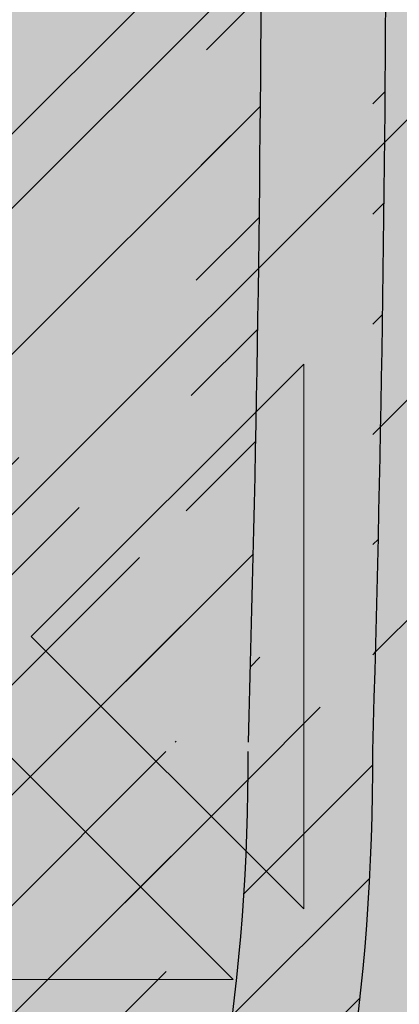
# Model space of a CAD drawing. Units: inches. Extents: x 844 to 2234, y 346 to 1084.
# Tile 11 of 93: x 1124.585 to 1125.555, y 691.183 to 693.702. Entities that reach past the tile are written whole.
import ezdxf

# ---------------------------------------------------------------- set-up
doc = ezdxf.new("R2010")
doc.units = ezdxf.units.IN
doc.header["$MEASUREMENT"] = 0
for name, color, linetype, lineweight in [('A-ANNO-DIMS', 2, 'Continuous', 18), ('furniture', 8, 'Continuous', 18), ('RA-AP-01$0$INT', 35, 'Continuous', 5)]:
    doc.layers.add(name, color=color, linetype=linetype, lineweight=lineweight)
doc.layers.add('RA-AP-01$0$FURN', color=3, linetype='Continuous')
doc.layers.add('RA-AP-01$0$WOOD', color=64, linetype='Continuous')
doc.styles.get("Standard").update_dxf_attribs({"font": 'arial.ttf'})
doc.dimstyles.get("Standard").update_dxf_attribs({"dimtxt": 6, "dimasz": 3, "dimexe": 0.18, "dimexo": 0.0625, "dimgap": 0.09, "dimtad": 0, "dimtih": 1, "dimtoh": 1, "dimdec": 1, "dimzin": 0, "dimdsep": 46, "dimlunit": 3, "dimtxsty": 'Standard', "dimblk": 'ARCHTICK', "dimcen": 0.09, "dimadec": 0, "dimazin": 0, "dimtfac": 1, "dimtdec": 1, "dimtofl": 0, "dimtmove": 0, "dimatfit": 3, "dimfxl": 1, "dimtolj": 1, "dimtzin": 0, "dimarcsym": 0})

# ---------------------------------------------------------------- blocks, each defined once
blk = doc.blocks.new('A$C18D01794')
at = {"layer": 'RA-AP-01$0$INT'}
h = blk.add_hatch(color=256, dxfattribs=at)
h.paths.add_polyline_path([(4.585917135068449, -6.356712009588271), (4.555206456959269, -6.35671200958746), (4.555206456959137, -6.387422687716308), (4.874495778835233, -6.706712009592356), (4.90520645695423, -6.676001331474049)])
h.paths.add_polyline_path([(5.255206456948813, -6.387422687716306), (5.255206456948682, -6.356712009605972), (5.224495778822613, -6.356712009605161), (4.905206456953498, -6.676001331474273), (4.935917135072151, -6.706712009592924)])
h.paths.add_polyline_path([(4.935917135072559, -6.706712009592068), (4.905206456953564, -6.737422687710376), (5.255206456951813, -7.087422687708613), (5.255206456951549, -7.026001331471008)])
h.paths.add_polyline_path([(4.555206456956399, -7.026001331471013), (4.555206456956134, -7.087422687708616), (4.905206456953821, -6.737422687710943), (4.874495778835166, -6.70671200959229)])
h = blk.add_hatch(color=256, dxfattribs=at)
h.paths.add_polyline_path([(4.585917135068448, -6.356712009588273), (4.614201406330596, -6.356712009589021), (4.668846067270487, -6.411356670531338), (4.723490728212344, -6.356712009591912), (4.771774999457151, -6.35671200959319), (4.826419660396886, -6.411356670535356), (4.862780050090322, -6.374996280843536), (4.844495778842715, -6.356712009595112), (4.862780050090411, -6.356712009595595), (4.905206456960182, -6.399138416468211), (4.947632863832445, -6.356712009597838), (4.965917135079675, -6.356712009598322), (4.947632863831759, -6.374996280845421), (4.983993253523576, -6.411356670538857), (5.038637914464627, -6.356712009600247), (5.08692218571208, -6.356712009601523), (5.141566846649976, -6.411356670541852), (5.196211507589851, -6.356712009604411), (5.224495778822615, -6.356712009605161), (4.905206456953975, -6.676001331473793)])
h.paths.add_polyline_path([(4.895206456956031, -6.637717060225675), (4.895206456958921, -6.528427738347902), (4.840561796018589, -6.583072399285802)], flags=16)
h.paths.add_polyline_path([(4.915206456955638, -6.637717060226121), (4.969851117895509, -6.583072399288678), (4.915206456957609, -6.528427738348344)], flags=16)
h.paths.add_polyline_path([(4.826419660395175, -6.568930263661755), (4.881064321335613, -6.514285602723745), (4.771774999456703, -6.514285602720857)], flags=16)
h.paths.add_polyline_path([(4.983993253519558, -6.568930263665262), (5.038637914460456, -6.514285602726792), (4.929348592581548, -6.514285602724816)], flags=16)
h.paths.add_polyline_path([(4.881064321336025, -6.494285602723742), (4.826419660397532, -6.439640941782821), (4.771774999457062, -6.494285602720859)], flags=16)
h.paths.add_polyline_path([(4.929348592582019, -6.494285602724817), (5.038637914460982, -6.494285602726792), (4.983993253522945, -6.439640941786327)], flags=16)
h.paths.add_polyline_path([(4.895206456960191, -6.480143467100443), (4.895206456962115, -6.407422687715913), (4.876922185715016, -6.389138416467584), (4.840561796021581, -6.425498806159401)], flags=16)
h.paths.add_polyline_path([(4.915206456958487, -6.480143467100889), (4.969851117899527, -6.425498806162279), (4.933490728206909, -6.389138416468043), (4.9152064569598, -6.40742268771434)], flags=16)
h.paths.add_polyline_path([(4.757632863832376, -6.480143467096812), (4.812277524772842, -6.425498806158772), (4.757632863834348, -6.370854145217844)], flags=16)
h.paths.add_polyline_path([(4.737632863832376, -6.480143467096286), (4.737632863834348, -6.370854145217375), (4.682988202893906, -6.425498806155385)], flags=16)
h.paths.add_polyline_path([(5.05278005008503, -6.480143467103376), (5.052780050087917, -6.370854145224413), (4.998135389146995, -6.425498806162908)], flags=16)
h.paths.add_polyline_path([(5.072780050085024, -6.480143467103744), (5.127424711025931, -6.42549880616527), (5.072780050087916, -6.370854145224832)], flags=16)
h.paths.add_polyline_path([(4.935917135072783, -6.706712009592292), (5.255206456948811, -6.387422687716309), (5.255206456948932, -6.415706958964177), (5.200561796010279, -6.470351619902839), (5.255206456949403, -6.524996280841948), (5.25520645694961, -6.5732805520894), (5.200561796009787, -6.627925213029239), (5.236922185702417, -6.664285602721864), (5.255206456949919, -6.646001331474357), (5.255206456949998, -6.664285602721898), (5.212780050078687, -6.706712009592262), (5.25520645695036, -6.749138416463932), (5.255206456950438, -6.767422687711313), (5.236922185702424, -6.749138416463297), (5.200561796009796, -6.785498806155928), (5.255206456950753, -6.840143467096874), (5.25520645695096, -6.888427738341682), (5.200561796010322, -6.943072399282328), (5.255206456951428, -6.997717060223427), (5.255206456951547, -7.026001331471006)])
h.paths.add_polyline_path([(5.042988202883395, -6.785498806155427), (5.097632863823085, -6.840143467095101), (5.097632863822622, -6.730854145216193)], flags=16)
h.paths.add_polyline_path([(5.028846067259663, -6.771356670531693), (5.083490728198774, -6.716712009592573), (4.974201406321001, -6.716712009593042)], flags=16)
h.paths.add_polyline_path([(5.117632863823087, -6.840143467095186), (5.172277524762331, -6.785498806155926), (5.11763286382262, -6.730854145216225)], flags=16)
h.paths.add_polyline_path([(5.08349072819877, -6.696712009593886), (5.028846067259652, -6.642067348654775), (4.974201406320998, -6.696712009593438)], flags=16)
h.paths.add_polyline_path([(5.131774999446817, -6.854285602718917), (5.186419660386065, -6.799640941779662), (5.241064321325782, -6.854285602719365)], flags=17)
h.paths.add_polyline_path([(5.131774999446228, -6.716712009592374), (5.186419660386065, -6.771356670532194), (5.222780050079488, -6.734996280838764), (5.204495778832781, -6.716712009592063)], flags=16)
h.paths.add_polyline_path([(5.097632863822613, -6.682569873970264), (5.097632863823061, -6.573280552091354), (5.042988202883383, -6.627925213031044)], flags=16)
h.paths.add_polyline_path([(5.131774999446899, -6.874285602718915), (5.241064321325809, -6.874285602719364), (5.186419660386591, -6.928930263658598)], flags=17)
h.paths.add_polyline_path([(5.131774999446226, -6.696712009594078), (5.204495778830767, -6.696712009594374), (5.22278005007868, -6.67842773834687), (5.186419660386049, -6.642067348654249)], flags=16)
h.paths.add_polyline_path([(5.11763286382262, -6.682569873970225), (5.17227752476232, -6.627925213030515), (5.117632863823064, -6.573280552091267)], flags=16)
h.paths.add_polyline_path([(5.186419660386069, -6.613783077405491), (5.241064321325754, -6.559138416465795), (5.131774999446791, -6.559138416466263)], flags=16)
h.paths.add_polyline_path([(5.131774999446872, -6.539138416466263), (5.24106432132578, -6.539138416465794), (5.186419660386554, -6.484493755526573)], flags=16)
h.paths.add_polyline_path([(5.255206456951811, -7.08742268770861), (5.255206456951895, -7.106712009588038), (4.555206456956052, -7.106712009588038), (4.555206456956136, -7.087422687708617), (4.905206456953973, -6.737422687710788)])
h.paths.add_polyline_path([(4.983993253513404, -6.8444937555241), (4.92934859257295, -6.899138416462108), (5.03863791445186, -6.899138416465014)], flags=16)
h.paths.add_polyline_path([(4.969851117889988, -6.83035161990006), (4.915206456952556, -6.775706958960171), (4.915206456949648, -6.884996280837944)], flags=16)
h.paths.add_polyline_path([(4.929348592572535, -6.919138416462105), (4.983993253511019, -6.973783077403037), (5.038637914451496, -6.919138416465012)], flags=16)
h.paths.add_polyline_path([(5.052780050074912, -6.93328055208906), (4.998135389134438, -6.987925213027088), (5.052780050072919, -7.042569873968025)], flags=16)
h.paths.add_polyline_path([(5.07278005007491, -6.933280552089588), (5.072780050072918, -7.042569873968497), (5.127424711013374, -6.987925213030498)], flags=16)
h.paths.add_polyline_path([(4.89520645695295, -6.775706958959721), (4.840561796013067, -6.830351619897157), (4.895206456950961, -6.884996280837494)], flags=16)
h.paths.add_polyline_path([(4.915206456948365, -6.933280552085403), (4.915206456946434, -7.006001331471951), (4.933490728192729, -7.024285602719066), (4.969851117886972, -6.987925213026453)], flags=16)
h.paths.add_polyline_path([(4.881064321327021, -6.899138416461022), (4.82641966038902, -6.84449375552057), (4.771774999448108, -6.899138416459029)], flags=16)
h.paths.add_polyline_path([(4.895206456950073, -6.933280552084951), (4.840561796009022, -6.987925213023558), (4.876922185700835, -7.024285602716997), (4.895206456948749, -7.006001331469487)], flags=16)
h.paths.add_polyline_path([(4.983993253510392, -7.0020673486505), (4.947632863816944, -7.038427738342319), (4.965917135064043, -7.05671200959023), (5.038637914448995, -7.056712009591555)], flags=16)
h.paths.add_polyline_path([(4.881064321326543, -6.91913841646102), (4.771774999447578, -6.919138416459031), (4.826419660385607, -6.973783077399508)], flags=16)
h.paths.add_polyline_path([(4.905206456946447, -7.014285602717636), (4.862780050074785, -7.056712009588352), (4.947632863816685, -7.056712009589775)], flags=16)
h.paths.add_polyline_path([(5.14156684663679, -7.002067348654549), (5.086922185696452, -7.056712009592438), (5.196211507574223, -7.056712009594425)], flags=16)
h.paths.add_polyline_path([(4.8264196603837, -7.002067348646972), (4.771774999442643, -7.056712009585575), (4.8444957788276, -7.056712009587508), (4.862780050075511, -7.038427738340416)], flags=16)
h.paths.add_polyline_path([(4.812277524760289, -6.98792521302292), (4.757632863822258, -6.933280552082447), (4.757632863819352, -7.042569873961408)], flags=16)
h.paths.add_polyline_path([(4.73763286382226, -6.933280552082079), (4.682988202881349, -6.987925213020536), (4.737632863819352, -7.04256987396099)], flags=16)
h.paths.add_polyline_path([(4.723490728195188, -7.056712009584289), (4.668846067257299, -7.002067348643949), (4.614201406317417, -7.056712009581383)], flags=16)
h.paths.add_polyline_path([(4.597632863829262, -6.706712009592262), (4.555206456957951, -6.664285602721896), (4.555206456958029, -6.646001331474357), (4.573490728205535, -6.664285602721864), (4.609851117898167, -6.627925213029238), (4.555206456958338, -6.573280552089402), (4.555206456958546, -6.524996280841952), (4.60985111789767, -6.470351619902839), (4.555206456959015, -6.415706958964177), (4.555206456959138, -6.387422687716309), (4.874495778835167, -6.70671200959229), (4.5552064569564, -7.026001331471015), (4.555206456956523, -6.997717060223433), (4.609851117897629, -6.94307239928233), (4.555206456956988, -6.888427738341681), (4.555206456957198, -6.840143467096881), (4.609851117898153, -6.78549880615593), (4.573490728205528, -6.749138416463297), (4.555206456957507, -6.76742268771132), (4.555206456957585, -6.749138416463933)])
h.paths.add_polyline_path([(4.712780050085332, -6.730854145216195), (4.712780050084863, -6.840143467095105), (4.767424711024555, -6.785498806155427)], flags=16)
h.paths.add_polyline_path([(4.726922185709173, -6.716712009592573), (4.781566846648288, -6.771356670531693), (4.836211507586949, -6.716712009593043)], flags=16)
h.paths.add_polyline_path([(4.692780050085327, -6.730854145216225), (4.638135389145619, -6.785498806155928), (4.692780050084865, -6.840143467095185)], flags=16)
h.paths.add_polyline_path([(4.726922185709182, -6.696712009593886), (4.836211507586949, -6.696712009593436), (4.7815668466483, -6.642067348654773)], flags=16)
h.paths.add_polyline_path([(4.678637914461726, -6.71671200959237), (4.605917135075169, -6.716712009592063), (4.587632863828464, -6.734996280838766), (4.623993253521887, -6.771356670532195)], flags=16)
h.paths.add_polyline_path([(4.712780050085336, -6.68256987397026), (4.767424711024568, -6.627925213031042), (4.71278005008489, -6.573280552091352)], flags=16)
h.paths.add_polyline_path([(4.678637914461726, -6.696712009594076), (4.623993253521899, -6.642067348654247), (4.587632863829271, -6.67842773834687), (4.605917135077185, -6.696712009594376)], flags=16)
h.paths.add_polyline_path([(4.692780050085336, -6.682569873970228), (4.692780050084889, -6.573280552091267), (4.638135389145632, -6.627925213030515)], flags=16)
h.paths.add_polyline_path([(4.623993253521885, -6.799640941779662), (4.678637914461131, -6.854285602718915), (4.56934859258217, -6.854285602719365)], flags=17)
h.paths.add_polyline_path([(4.623993253521901, -6.613783077405509), (4.678637914461158, -6.559138416466263), (4.569348592582195, -6.559138416465795)], flags=16)
h.paths.add_polyline_path([(4.678637914461051, -6.874285602718915), (4.623993253521361, -6.928930263658598), (4.569348592582143, -6.874285602719364)], flags=17)
h.paths.add_polyline_path([(4.678637914461076, -6.539138416466263), (4.623993253521399, -6.484493755526573), (4.569348592582167, -6.539138416465796)], flags=16)
h = blk.add_hatch(color=256, dxfattribs=at)
h.paths.add_polyline_path([(5.028846067259997, -6.642067348655121), (4.974201406321342, -6.696712009593783), (5.083490728199115, -6.69671200959423)])
h.paths.add_polyline_path([(4.974201406321344, -6.716712009593388), (5.028846067260004, -6.771356670532039), (5.083490728199117, -6.716712009592919)])
h.paths.add_polyline_path([(5.042988202883738, -6.785498806155768), (5.097632863823428, -6.840143467095449), (5.097632863822963, -6.73085414521654)])
h.paths.add_polyline_path([(5.117632863822961, -6.730854145216568), (5.117632863823428, -6.840143467095531), (5.172277524762674, -6.785498806156272)])
h.paths.add_polyline_path([(5.131774999446572, -6.716712009592718), (5.186419660386406, -6.77135667053254), (5.222780050079831, -6.734996280839116), (5.204495778833122, -6.716712009592409)])
h.paths.add_polyline_path([(5.236922185702764, -6.749138416463644), (5.200561796010139, -6.785498806156274), (5.255206456949971, -6.840143467096101), (5.255206456950271, -6.76742268771115)])
h.paths.add_polyline_path([(5.186419660386412, -6.799640941780006), (5.131774999447164, -6.854285602719262), (5.241064321326123, -6.854285602719711)])
h.paths.add_polyline_path([(5.131774999447238, -6.874285602719261), (5.186419660386934, -6.928930263658944), (5.241064321326153, -6.874285602719709)])
h.paths.add_polyline_path([(5.200561796010663, -6.943072399282675), (5.255206456949324, -6.997717060221329), (5.255206456949777, -6.888427738343558)])
h.paths.add_polyline_path([(5.21278005007903, -6.706712009592607), (5.255206456950223, -6.749138416463798), (5.255206456950696, -6.664285602721891)])
h.paths.add_polyline_path([(5.13177499944657, -6.696712009594424), (5.204495778831106, -6.696712009594723), (5.222780050079024, -6.678427738347219), (5.186419660386397, -6.642067348654592)])
h.paths.add_polyline_path([(5.117632863823405, -6.573280552091611), (5.117632863822955, -6.682569873970578), (5.172277524762665, -6.627925213030859)])
h.paths.add_polyline_path([(5.042988202883727, -6.627925213031387), (5.097632863822957, -6.682569873970603), (5.097632863823407, -6.573280552091697)])
h.paths.add_polyline_path([(5.131774999447135, -6.559138416466609), (5.186419660386394, -6.613783077405857), (5.241064321326097, -6.559138416466144)])
h.paths.add_polyline_path([(5.200561796010128, -6.627925213029584), (5.236922185702758, -6.664285602722211), (5.255206456950264, -6.646001331474705), (5.255206456949948, -6.573280552089752)])
h.paths.add_polyline_path([(5.186419660386895, -6.484493755526919), (5.131774999447213, -6.539138416466609), (5.241064321326127, -6.539138416466142)])
h.paths.add_polyline_path([(5.200561796010624, -6.470351619903183), (5.255206456949745, -6.524996280842298), (5.255206456949276, -6.415706958964523)])
for p, q in [((4.935917135072783, -6.706712009592292), (5.255206456951548, -7.026001331471007)), ((5.083490728198772, -6.716712009592574), (4.974201406321001, -6.716712009593042)), ((5.08349072819877, -6.716712009592578), (5.028846067259663, -6.771356670531693)), ((5.09763286382262, -6.730854145216195), (5.042988202883395, -6.785498806155425)), ((5.097632863823085, -6.840143467095105), (5.09763286382262, -6.730854145216195)), ((4.905206456953975, -6.737422687710788), (5.255206456951811, -7.087422687708611)), ((5.042988202883397, -6.785498806155427), (5.097632863823085, -6.840143467095105))]:
    blk.add_line(p, q, dxfattribs=at)
blk = doc.blocks.new('A$C32926AE1')
at = {"layer": 'RA-AP-01$0$FURN'}
h = blk.add_hatch(dxfattribs=at)
h.set_pattern_fill('ANSI31', color=256, scale=0.1, style=0)
h.set_pattern_definition([(45, (0, 0), (-0.0088388347648318, 0.0088388347648318), [])])
edge = h.paths.add_edge_path(flags=16)
edge.add_arc((4.904771284329206, 4.246793130718756), 0.2603971832811541, 75.22398030683196, 104.7760196931204)
edge.add_arc((4.904771284329206, 4.246793130718756), 0.2603971832811541, 75.223980306832, 104.77601969312039, ccw=False)
edge = h.paths.add_edge_path(flags=16)
edge.add_arc((4.904771284329206, 4.067062675376612), 0.2603971832811541, 255.2239803068796, 284.776019693168)
edge.add_arc((4.904771284329206, 4.067062675376612), 0.2603971832811541, 255.22398030687958, 284.77601969316805, ccw=False)
edge = h.paths.add_edge_path(flags=0)
edge.add_arc((4.904771284329206, 4.067062675376612), 0.2603971832811541, 255.2239803068796, 284.776019693168)
edge.add_arc((4.904771284329206, 4.067062675376612), 0.2603971832811541, 255.22398030687958, 284.77601969316805, ccw=False)
edge = h.paths.add_edge_path(flags=0)
edge.add_arc((4.904771284329206, 4.067062675376612), 0.2603971832811541, 255.2239803068796, 284.776019693168)
edge.add_arc((4.904771284329206, 4.067062675376612), 0.2603971832811541, 255.22398030687958, 284.77601969316805, ccw=False)
edge = h.paths.add_edge_path()
edge.add_arc((4.604388392048174, 4.588829985554312), 0.1599999999999918, 342.3781640246255, 354.4317409793762)
edge.add_arc((5.090145208887507, 4.43216705527679), 0.3503971832811637, 162.0091218307731, 180.3186872093483)
edge.add_arc((5.205154176610243, 4.588829985554953), 0.1599999999999917, 185.5682590208461, 197.6218359767349)
edge.add_arc((4.904771284329229, 4.246793130718735), 0.3503971832811761, 72.00912183053516, 107.9908781690354)
edge.add_arc((9.535952835716557, 4.28682295566602), 4.798342501046485, 178.2875002453811, 181.5576802719453)
edge.add_arc((4.719397359771122, 4.43216705527679), 0.3503971832811637, 359.6813127906516, 377.9908781692269)
edge.add_arc((9.535967292294904, 4.286822350292874), 4.778371420254705, 178.2965938931842, 181.5667745797229)
edge.add_arc((4.719397359771122, 4.43216705527679), 0.3303971832811637, 359.6813127906516, 377.9908781692269)
edge.add_arc((0.2735752763637294, 4.286822350292874), 4.7783714202547, 358.4332254202771, 361.7034061068158)
edge.add_arc((5.061434214606998, 4.732549947558029), 0.1600000000000254, 252.3781640250584, 264.4317409792362)
edge.add_arc((4.748108354051257, 4.732549947558012), 0.1600000000000541, 275.5682590208426, 287.6218359759532)
edge.add_arc((4.604388392048115, 4.588829985554317), 0.1800000000000505, 342.3567572500182, 349.3735009646207)
edge.add_arc((5.205154176610254, 4.588829985554976), 0.1800000000000069, 190.6264990356027, 197.6432427513933)
edge.add_arc((5.061434214607106, 4.732549947558013), 0.1800000000000424, 252.3567572496606, 259.3735009644582)
edge.add_arc((4.904771284329208, 4.246793130718737), 0.3303971832811676, 71.99844483668534, 108.0015551637021)
edge.add_arc((4.748108354051414, 4.732549947558045), 0.1800000000000547, 280.6264990355479, 287.6432427495938)
edge.add_arc((5.090145208887514, 4.432167055276789), 0.2803971832811691, 162.8706300666893, 180.816523289902)
edge.add_arc((4.719397359771136, 4.432167055276689), 0.2803971832811534, 359.183476710103, 377.1293699333214)
edge.add_arc((4.904771284329222, 4.246793130718737), 0.2803971832811769, 72.87063006672916, 107.1293699332334)
edge.add_arc((5.090145208887522, 4.432167055276788), 0.2603971832811776, 165.2239803068007, 180.9953123810312)
edge.add_arc((4.719397359771141, 4.432167055276699), 0.2603971832811458, 359.0046876189768, 374.7760196932087)
edge.add_arc((5.090145208887507, 4.43216705527679), 0.3303971832811637, 162.0091218307731, 180.3186872093483)
edge.add_arc((9.53595427642584, 4.285015535491528), 4.728345371032053, 178.265043920078, 181.5679956281801)
edge.add_arc((0.2735882922327999, 4.285015535491582), 4.728345371032045, 358.4320043718193, 361.7349560799204)
edge.add_arc((9.535953591267507, 4.284458026472751), 4.708343996644348, 178.2573054306777, 181.5704995759608)
edge.add_arc((0.273588977391114, 4.284458026472785), 4.708343996644358, 358.4295004240388, 361.7426945693213)
edge.add_arc((0.2735889773911131, 4.029397779622582), 4.708343996644359, 358.2573054306787, 361.5704995759613)
edge.add_arc((9.535953591267518, 4.029397779622618), 4.708343996644359, 178.4295004240391, 181.7426945693223)
edge.add_arc((0.2735882922327901, 4.028840270603786), 4.728345371032054, 358.2650439200796, 361.5679956281808)
edge.add_arc((9.53595427642584, 4.028840270603841), 4.728345371032054, 178.4320043718199, 181.7349560799219)
edge.add_arc((0.2735752763637302, 4.027033455802493), 4.778371420254699, 358.2965938931842, 361.5667745797229)
edge.add_arc((4.719397359771122, 3.881688750818578), 0.3303971832811637, 342.0091218307731, 360.3186872093484)
edge.add_arc((5.090145208887507, 3.881688750818578), 0.3303971832811637, 179.6813127906516, 197.9908781692269)
edge.add_arc((9.535967292294904, 4.027033455802493), 4.778371420254705, 178.433225420277, 181.7034061068158)
edge.add_arc((4.719397359771122, 3.881688750818578), 0.3503971832811637, 342.0091218307731, 360.3186872093484)
edge.add_arc((9.53595283571655, 4.027032850429349), 4.79834250104648, 178.4423197280546, 181.7124997546188)
edge.add_arc((4.719397359771141, 3.881688750818669), 0.2603971832811458, 345.2239803067913, 360.9953123810232)
edge.add_arc((5.090145208887522, 3.88168875081858), 0.2603971832811776, 179.0046876189687, 194.7760196931993)
edge.add_arc((4.904771284329222, 4.067062675376631), 0.2803971832811769, 252.8706300667665, 287.1293699332708)
edge.add_arc((4.719397359771136, 3.881688750818678), 0.2803971832811534, 342.8706300666787, 360.8165232898969)
edge.add_arc((5.090145208887514, 3.881688750818579), 0.2803971832811691, 179.183476710098, 197.1293699333106)
edge.add_arc((4.748108354051414, 3.581305858537323), 0.1800000000000547, 72.3567572504062, 79.37350096445199)
edge.add_arc((4.904771284329208, 4.067062675376631), 0.3303971832811676, 251.9984448362979, 288.0015551633146)
edge.add_arc((5.061434214607106, 3.581305858537355), 0.1800000000000424, 100.6264990355418, 107.6432427503394)
edge.add_arc((5.205154176610254, 3.725025820540392), 0.1800000000000069, 162.3567572486066, 169.3735009643972)
edge.add_arc((4.604388392048115, 3.725025820541051), 0.1800000000000505, 10.62649903537925, 17.64324274998182)
edge.add_arc((4.748108354051257, 3.581305858537356), 0.1600000000000541, 72.37816402404681, 84.43174097915735)
edge.add_arc((4.904771284329229, 4.067062675376632), 0.3503971832811761, 252.0091218309645, 287.9908781694648)
edge.add_arc((5.061434214606998, 3.581305858537339), 0.1600000000000254, 95.56825902076373, 107.6218359749416)
edge.add_arc((5.205154176610243, 3.725025820540414), 0.1599999999999917, 162.3781640232651, 174.4317409791539)
edge.add_arc((5.090145208887507, 3.881688750818578), 0.3503971832811637, 179.6813127906516, 197.9908781692269)
edge.add_arc((4.604388392048174, 3.725025820541056), 0.1599999999999918, 5.568259020623824, 17.62183597537444)
edge.add_arc((0.2735897329420762, 4.28682295566602), 4.798342501046482, 358.4423197280547, 361.7124997546188)
edge.add_arc((0.2735897329420691, 4.027032850429348), 4.798342501046489, 358.2875002453812, 361.5576802719453)
at = {"layer": 'RA-AP-01$0$WOOD'}
h = blk.add_hatch(color=256, dxfattribs=at)
h.dxf.hatch_style = 1
h.paths.add_polyline_path([(5.157430609644524, 4.573483066760929, -0.1009492694046607), (5.155401577623758, 4.593365984175333, -0.1842662638101597), (5.172249623284174, 4.638795604568598, 0.2056608120311276), (5.179560981299304, 4.661316324430096, 0.3614336704623542), (5.134352340494423, 4.706524965234944, 0.2056608120311297), (5.111831620632933, 4.699213607219793, -0.1842662638101113), (5.066402000239693, 4.682365561559342, -0.1055311479399994), (5.045656153913092, 4.68467289944697, 0.1567636581983829), (4.763886414745334, 4.684672899446966, -0.1055311479399895), (4.743140568418733, 4.68236556155934, -0.1842662638100833), (4.6977109480255, 4.69921360721979, 0.2056608120302612), (4.675190228164109, 4.706524965234949, 0.3614336704708441), (4.629981587358889, 4.66131632442871, 0.2056608120245944), (4.637292945374126, 4.638795604567974, -0.1842662638101024), (4.654140991034615, 4.59336598417475, -0.1009492694055169), (4.652111959013835, 4.573483066760181, 0.021410119221476), (4.629748025606143, 4.156712009541676, 0.0214101192214795), (4.652111959013809, 3.739940952323101, -0.1009492694059586), (4.654140991034615, 3.720058034908448, -0.1842662638100975), (4.637292945374126, 3.674628414515226, 0.2056608120245705), (4.629981587358889, 3.652107694654492, 0.3614336704708879), (4.675190228164113, 3.606899053848249, 0.2056608120302384), (4.697710948025501, 3.614210411863408, -0.1842662638100995), (4.743140568418738, 3.63105845752386, -0.1055311479402541), (4.763886414745388, 3.628751119636215, 0.1567636581983776), (5.045656153913137, 3.628751119636244, -0.1055311479397538), (5.066402000239692, 3.631058457523857, -0.1842662638101067), (5.111831620632931, 3.614210411863407, 0.2056608120310924), (5.134352340494417, 3.606899053848256, 0.3614336704624001), (5.179560981299307, 3.652107694653103, 0.2056608120311314), (5.172249623284175, 3.6746284145146, -0.1842662638101402), (5.155401577623758, 3.72005803490786, -0.1009492694051366), (5.15743060964455, 3.739940952322354, 0.0214101192215073), (5.179794543052287, 4.156712009541468, 0.0214101192215252)])
h.paths.add_polyline_path([(4.639748609479751, 4.156712009541513, 0.0213537860821624), (4.661970494867118, 3.741887061152232, -0.094075836301374), (4.664143710413708, 3.7196126951003, -0.1824818158568985), (4.644813765429836, 3.668037719127816, 0.2056608120245319), (4.639939526753007, 3.653023905887301, 0.3614336704710246), (4.676106439397173, 3.616856993242342, 0.2056608120302234), (4.691120252638095, 3.621731231919122, -0.1824818158602558), (4.742695228611606, 3.641061176902986, -0.1029891339458722), (4.766991894714349, 3.638256818950944, 0.156709409989566), (5.042550673941472, 3.638256818950105, -0.102989133958497), (5.066847340047078, 3.641061176902949, -0.1824818158594995), (5.118422316020358, 3.621731231919103, 0.2056608120311416), (5.133436129261316, 3.616856993242346, 0.3614336704621468), (5.169603041905217, 3.653023905886178, 0.2056608120310986), (5.164728803228477, 3.668037719127177, -0.1824818158565612), (5.145398858244737, 3.719612695099578, -0.0940758363009313), (5.147572073791232, 3.741887061151398, 0.0213537860822023), (5.169793959178681, 4.156712009541451, 0.0213537860822226), (5.147572073791203, 4.571536957931898, -0.0940758363005034), (5.145398858244737, 4.59381132398362, -0.1824818158565587), (5.164728803228476, 4.645386299956021, 0.2056608120311045), (5.169603041905216, 4.66040011319702, 0.3614336704621845), (5.133436129261313, 4.696567025840856, 0.2056608120310773), (5.118422316020359, 4.691692787164098, -0.182481815859508), (5.066847340047078, 4.67236284218025, -0.1029891339584606), (5.04255067394148, 4.675167200133092, 0.156709409989566), (4.766991894714357, 4.675167200132257, -0.1029891339458842), (4.742695228611611, 4.672362842180213, -0.1824818158602725), (4.691120252638095, 4.691692787164077, 0.2056608120302152), (4.676106439397174, 4.696567025840858, 0.3614336704710363), (4.639939526753005, 4.660400113195899, 0.2056608120245495), (4.644813765429837, 4.645386299955384, -0.1824818158568934), (4.664143710413708, 4.593811323982902, -0.0940758363009187), (4.661970494867149, 4.571536957931074, 0.021353786082177)], flags=16)
h.paths.add_polyline_path([(5.129794543052235, 4.432167055276933, -0.0141661062790638), (5.130152669293814, 4.156927903047693, -0.0141661062790647), (5.129794543052234, 3.881688750818433, -0.0785247771143638), (5.10979738006795, 3.755143611847103, 0.0945969212073497), (5.105408519571111, 3.717898134952927, 0.1043170707844957), (5.116074640131521, 3.670385395016088, 0.1043170707864965), (5.068561900193738, 3.681051515576561, 0.09459692119553), (5.031316423304057, 3.676662655080835, -0.1580239521427272), (4.778226145355827, 3.676662655080367, 0.0945969211986668), (4.740980668464973, 3.681051515576592, 0.1043170707882822), (4.693467928526415, 3.670385395015844, 0.1043170707867916), (4.704134049087309, 3.717898134953662, 0.0945969211972894), (4.69974518859162, 3.755143611844042, -0.0785247771163196), (4.679748025606343, 3.881688750818406, -0.0141661062790663), (4.679389899364763, 4.156927903047693, -0.0141661062790672), (4.679748025606343, 4.432167055276998, -0.0785247771163064), (4.699745188591625, 4.55871219425134, 0.094596921197333), (4.704134049087308, 4.595957671141738, 0.1043170707867205), (4.693467928526416, 4.643470411079523, 0.1043170707882628), (4.740980668464965, 4.632804290518776, 0.0945969211988114), (4.778226145355874, 4.637193151015016, -0.158023952142669), (5.031316423304015, 4.637193151014546, 0.0945969211956361), (5.068561900193736, 4.632804290518806, 0.1043170707864979), (5.11607464013152, 4.643470411079278, 0.1043170707844617), (5.105408519571112, 4.595957671142455, 0.0945969212074597), (5.109797380067959, 4.558712194248236, -0.0785247771143467)], flags=0)
h.paths.add_polyline_path([(5.119794532311105, 4.432259799204851, -0.0142000800617244), (5.120156169157484, 4.156927903047701, -0.0142000800617277), (5.119794532311105, 3.881596006890482, -0.0784894509520253), (5.100273383573699, 3.758192358677797, 0.0940138827242913), (5.095413455884425, 3.717477693979438, 0.0606271852308753), (5.099615656341024, 3.686844378806616, 0.0606271852322524), (5.068982341167493, 3.691046579263239, 0.0940138827010453), (5.028267676478798, 3.686186651576848, -0.1580706864508061), (4.781274892180912, 3.686186651576435, 0.0940138827026903), (4.740560227491556, 3.691046579263279, 0.0606271852339895), (4.709926912317155, 3.686844378806508, 0.0606271852329405), (4.714129112773991, 3.717477693980356, 0.094013882701304), (4.709269185087677, 3.758192358669163, -0.0784894509577193), (4.689748036347473, 3.881596006890469, -0.014200080061729), (4.689386399501094, 4.156927903047709, -0.0142000800617217), (4.689748036347473, 4.432259799204808, -0.078489450957724), (4.709269185087651, 4.555663447426125, 0.0940138827014585), (4.714129112773992, 4.596378112114996, 0.0606271852329731), (4.709926912317154, 4.62701142728886, 0.0606271852340196), (4.74056022749157, 4.622809226832087, 0.0940138827024997), (4.781274892180847, 4.627669154518912, -0.1580706864508359), (5.028267676478777, 4.627669154518526, 0.0940138827010946), (5.068982341167492, 4.622809226832129, 0.060627185232254), (5.099615656341024, 4.627011427288751, 0.0606271852308727), (5.095413455884425, 4.59637811211593, 0.0940138827241088), (5.100273383573675, 4.555663447417647, -0.0784894509520978)], flags=0)
h.paths.add_polyline_path([(5.06978912287499, 4.430218106756144, -0.014241683694547), (5.070173729147532, 4.156927903047672, -0.0142416836945458), (5.06978912287499, 3.883637699339223, -0.0800609523125196), (5.052662118612511, 3.773463122773442, 0.0526421978001116), (5.04590916754064, 3.740550867606997, 0.0526421977992423), (5.012996912374707, 3.73379791653534, -0.1583028414718258), (4.796545656286308, 3.73379791653451, 0.0526421978034211), (4.763633401117837, 3.740550867607021, 0.0526421978018622), (4.756880450045755, 3.773463122774558, -0.0800609523117106), (4.739753445783639, 3.883637699339268, -0.0142416836945435), (4.739368839511098, 4.156927903047671, -0.0142416836945477), (4.739753445783639, 4.430218106756155, -0.0800609523116345), (4.75688045004574, 4.540392683320762, 0.052642197801941), (4.763633401117837, 4.573304938488346, 0.0526421978035071), (4.796545656286361, 4.580057889560873, -0.1583028414717561), (5.012996912374669, 4.580057889560039, 0.0526421977993048), (5.04590916754064, 4.57330493848837, 0.0526421978002057), (5.052662118612529, 4.540392683321868, -0.080060952312477)], flags=0)
h.paths.add_polyline_path([(5.049789715110557, 4.43038092723357, -0.0143097550741839), (5.05018085590259, 4.156927903047715, -0.0143097550741854), (5.049789715110558, 3.883474878861827, -0.0800685599149176), (5.03362098255317, 3.779581877367999, 0.0306258898956367), (5.028241146483733, 3.758218888663947, 0.0306258898977031), (5.006878157778253, 3.75283905259408, -0.1583983521624096), (4.802664410878162, 3.752839052594731, 0.0306258898946014), (4.781301422174808, 3.758218888663924, 0.0306258898967912), (4.775921586105202, 3.779581877368794, -0.080068559914251), (4.759752853548071, 3.883474878861786, -0.0143097550741854), (4.759361712756037, 4.156927903047671, -0.0143097550741854), (4.759752853548071, 4.430380927233557, -0.0800685599142479), (4.775921586105193, 4.534273928726546, 0.0306258898968306), (4.781301422174808, 4.555636917431444, 0.0306258898945754), (4.802664410878143, 4.561016753500631, -0.1583983521624168), (5.006878157778244, 4.561016753501291, 0.0306258898977177), (5.028241146483733, 4.555636917431421, 0.0306258898958182), (5.03362098255321, 4.534273928727244, -0.080068559914796)], flags=0)
h.paths.add_polyline_path([(4.999766070382627, 4.428171244713864, -0.0143443147609634), (5.000198441819402, 4.156927903047689, -0.0143443147609612), (4.999766070382627, 3.885684561381556, -0.0784641635803329), (4.987356730658798, 3.799103304488872, -0.1506053783831347), (4.822185837999821, 3.79910330448882, -0.0784641635803318), (4.809776498276007, 3.885684561381509, -0.014344314760963), (4.809344126839227, 4.156927903047677, -0.0143443147609645), (4.809776498276007, 4.428171244713873, -0.0784641635803192), (4.822185837999822, 4.514752501606549, -0.1506053783831338), (4.987356730658798, 4.514752501606494, -0.078464163580285)], flags=0)
h.paths.add_polyline_path([(4.979755254238824, 4.42764379880488, -0.0143772539198268), (4.980205517789977, 4.156927903047693, -0.0143772539198275), (4.979755254238824, 3.886212007290489, -0.0689242507424422), (4.971183264704897, 3.815276770442801, -0.1296645318904179), (4.838359303953726, 3.815276770442746, -0.0689242507424186), (4.829787314419809, 3.886212007290419, -0.0143772539198292), (4.829337050868653, 4.156927903047653, -0.0143772539198325), (4.829787314419809, 4.427643798804946, -0.0689242507424211), (4.838359303953725, 4.498579035652621, -0.1296645318904187), (4.971183264704897, 4.498579035652565, -0.0689242507424401)], flags=0)
h = blk.add_hatch(color=256, dxfattribs=at)
h.dxf.hatch_style = 1
h.paths.add_polyline_path([(5.145398858244737, 4.59381132398362, -0.1824818158565616), (5.164728803228476, 4.645386299956021, 0.2056608120311045), (5.169603041905216, 4.66040011319702, 0.3614336704621845), (5.133436129261313, 4.696567025840856, 0.2056608120310773), (5.118422316020359, 4.691692787164098, -0.182481815859508), (5.066847340047078, 4.67236284218025, -0.1029891339584606), (5.04255067394148, 4.675167200133092, 0.156709409989566), (4.766991894714357, 4.675167200132257, -0.1029891339458842), (4.742695228611611, 4.672362842180213, -0.1824818158602725), (4.691120252638095, 4.691692787164077, 0.2056608120302152), (4.676106439397174, 4.696567025840858, 0.3614336704710363), (4.639939526753005, 4.660400113195899, 0.2056608120245495), (4.644813765429837, 4.645386299955384, -0.1824818158568934), (4.664143710413708, 4.593811323982902, -0.0940758363009187), (4.661970494867149, 4.571536957931074, 0.0213537860821772), (4.639748609479751, 4.156712009541507, 0.0213537860821625), (4.661970494867119, 3.741887061152226, -0.0940758363013071), (4.664143710413708, 3.719612695100309, -0.1824818158569294), (4.644813765429836, 3.668037719127816, 0.2056608120245319), (4.639939526753007, 3.653023905887301, 0.3614336704710246), (4.676106439397173, 3.616856993242342, 0.2056608120302234), (4.691120252638095, 3.621731231919122, -0.1824818158602558), (4.742695228611606, 3.641061176902986, -0.1029891339458722), (4.766991894714349, 3.638256818950944, 0.156709409989566), (5.042550673941472, 3.638256818950105, -0.102989133958497), (5.066847340047078, 3.641061176902949, -0.1824818158594995), (5.118422316020358, 3.621731231919103, 0.2056608120311416), (5.133436129261316, 3.616856993242346, 0.3614336704621468), (5.169603041905217, 3.653023905886178, 0.2056608120310986), (5.164728803228477, 3.668037719127177, -0.1824818158565612), (5.145398858244737, 3.719612695099578, -0.0940758363009313), (5.147572073791232, 3.741887061151398, 0.0213537860822023), (5.169793959178681, 4.156712009541451, 0.0213537860822226), (5.147572073791203, 4.571536957931898, -0.0940758363004996)])
h.paths.add_polyline_path([(5.109797380067958, 4.55871219424824, -0.0785247771143472), (5.129794543052234, 4.432167055276936, -0.0141661062790644), (5.130152669293814, 4.156927903047685, -0.014166106279066), (5.129794543052234, 3.881688750818401, -0.0785247771143517), (5.109797380067946, 3.755143611847092, 0.0945969212073132), (5.105408519571111, 3.717898134952929, 0.1043170707844995), (5.116074640131521, 3.670385395016088, 0.1043170707864965), (5.068561900193738, 3.681051515576561, 0.09459692119553), (5.031316423304057, 3.676662655080835, -0.1580239521427272), (4.778226145355827, 3.676662655080367, 0.0945969211986668), (4.740980668464973, 3.681051515576592, 0.1043170707882822), (4.693467928526415, 3.670385395015844, 0.1043170707867916), (4.704134049087309, 3.717898134953662, 0.0945969211972894), (4.69974518859162, 3.755143611844042, -0.0785247771163196), (4.679748025606343, 3.881688750818406, -0.0141661062790663), (4.679389899364763, 4.156927903047693, -0.0141661062790672), (4.679748025606343, 4.432167055276998, -0.0785247771163064), (4.699745188591625, 4.55871219425134, 0.094596921197333), (4.704134049087308, 4.595957671141738, 0.1043170707867205), (4.693467928526416, 4.643470411079523, 0.1043170707882628), (4.740980668464965, 4.632804290518776, 0.0945969211988114), (4.778226145355874, 4.637193151015016, -0.158023952142669), (5.031316423304015, 4.637193151014546, 0.0945969211956361), (5.068561900193736, 4.632804290518806, 0.1043170707864979), (5.11607464013152, 4.643470411079278, 0.1043170707844617), (5.105408519571112, 4.595957671142455, 0.0945969212074504)], flags=16)
h.paths.add_polyline_path([(5.100273383573655, 4.55566344741771, -0.0784894509521388), (5.119794532311105, 4.432259799204852, -0.0142000800617252), (5.120156169157484, 4.156927903047686, -0.014200080061726), (5.119794532311105, 3.881596006890502, -0.0784894509520446), (5.100273383573696, 3.758192358677786, 0.0940138827242721), (5.095413455884425, 3.717477693979436, 0.0606271852308692), (5.099615656341024, 3.686844378806616, 0.0606271852322522), (5.068982341167493, 3.691046579263239, 0.0940138827010453), (5.028267676478798, 3.686186651576848, -0.1580706864508061), (4.781274892180912, 3.686186651576435, 0.0940138827026903), (4.740560227491556, 3.691046579263279, 0.0606271852339895), (4.709926912317155, 3.686844378806508, 0.0606271852329405), (4.714129112773991, 3.717477693980356, 0.094013882701304), (4.709269185087677, 3.758192358669163, -0.0784894509577193), (4.689748036347473, 3.881596006890469, -0.014200080061729), (4.689386399501094, 4.156927903047709, -0.0142000800617217), (4.689748036347473, 4.432259799204808, -0.078489450957724), (4.709269185087651, 4.555663447426125, 0.0940138827014585), (4.714129112773992, 4.596378112114996, 0.0606271852329731), (4.709926912317154, 4.62701142728886, 0.0606271852340196), (4.74056022749157, 4.622809226832087, 0.0940138827024997), (4.781274892180847, 4.627669154518912, -0.1580706864508359), (5.028267676478777, 4.627669154518526, 0.0940138827010946), (5.068982341167492, 4.622809226832129, 0.060627185232254), (5.099615656341024, 4.627011427288751, 0.0606271852308727), (5.095413455884425, 4.59637811211593, 0.094013882723957)], flags=0)
h.paths.add_polyline_path([(5.04590916754064, 4.57330493848837, 0.0526421978002057), (5.052662118612529, 4.540392683321868, -0.0800609523124783), (5.06978912287499, 4.430218106756142, -0.0142416836945469), (5.070173729147532, 4.156927903047672, -0.0142416836945458), (5.06978912287499, 3.883637699339223, -0.0800609523125196), (5.052662118612511, 3.773463122773442, 0.0526421978001116), (5.04590916754064, 3.740550867606997, 0.0526421977992423), (5.012996912374707, 3.73379791653534, -0.1583028414718258), (4.796545656286308, 3.73379791653451, 0.0526421978034211), (4.763633401117837, 3.740550867607021, 0.0526421978018622), (4.756880450045755, 3.773463122774558, -0.0800609523117106), (4.739753445783639, 3.883637699339268, -0.0142416836945435), (4.739368839511098, 4.156927903047671, -0.0142416836945477), (4.739753445783639, 4.430218106756155, -0.0800609523116345), (4.75688045004574, 4.540392683320762, 0.052642197801941), (4.763633401117837, 4.573304938488346, 0.0526421978035071), (4.796545656286361, 4.580057889560873, -0.1583028414717561), (5.012996912374669, 4.580057889560039, 0.0526421977993048)], flags=0)
h.paths.add_polyline_path([(5.028241146483733, 4.555636917431422, 0.0306258898956949), (5.033620982553182, 4.534273928727329, -0.0800685599148649), (5.049789715110557, 4.430380927233569, -0.0143097550741839), (5.05018085590259, 4.156927903047715, -0.0143097550741854), (5.049789715110558, 3.883474878861827, -0.0800685599149176), (5.03362098255317, 3.779581877367999, 0.0306258898956367), (5.028241146483733, 3.758218888663947, 0.0306258898977031), (5.006878157778253, 3.75283905259408, -0.1583983521624096), (4.802664410878162, 3.752839052594731, 0.0306258898946014), (4.781301422174808, 3.758218888663924, 0.0306258898967912), (4.775921586105202, 3.779581877368794, -0.080068559914251), (4.759752853548071, 3.883474878861786, -0.0143097550741854), (4.759361712756037, 4.156927903047671, -0.0143097550741854), (4.759752853548071, 4.430380927233557, -0.0800685599142479), (4.775921586105193, 4.534273928726546, 0.0306258898968306), (4.781301422174808, 4.555636917431444, 0.0306258898945754), (4.802664410878143, 4.561016753500631, -0.1583983521624168), (5.006878157778244, 4.561016753501291, 0.0306258898977174)], flags=0)
h.paths.add_polyline_path([(4.987356730658798, 4.514752501606494, -0.0784641635803018), (4.999766070382627, 4.428171244713845, -0.0143443147609637), (5.000198441819402, 4.156927903047665, -0.0143443147609622), (4.999766070382628, 3.885684561381514, -0.0784641635802952), (4.987356730658797, 3.799103304488872, -0.1506053783831338), (4.822185837999821, 3.799103304488819, -0.0784641635803342), (4.809776498276007, 3.885684561381512, -0.0143443147609628), (4.809344126839227, 4.156927903047676, -0.0143443147609646), (4.809776498276007, 4.428171244713873, -0.0784641635803192), (4.822185837999822, 4.514752501606549, -0.1506053783831338)], flags=0)
h.paths.add_polyline_path([(4.971183264704897, 4.498579035652566, -0.0689242507424384), (4.979755254238824, 4.427643798804883, -0.0143772539198276), (4.980205517789977, 4.15692790304768, -0.0143772539198258), (4.979755254238823, 3.88621200729051, -0.0689242507424628), (4.971183264704897, 3.815276770442801, -0.129664531890417), (4.838359303953726, 3.815276770442746, -0.0689242507424186), (4.829787314419809, 3.886212007290419, -0.0143772539198292), (4.829337050868653, 4.156927903047653, -0.0143772539198325), (4.829787314419809, 4.427643798804946, -0.0689242507424211), (4.838359303953725, 4.498579035652621, -0.1296645318904187)], flags=0)
h = blk.add_hatch(dxfattribs=at)
h.set_pattern_fill('ANSI31', color=256, scale=0.05, style=0)
h.set_pattern_definition([(45, (0, 0), (-0.0044194173824159, 0.0044194173824159), [])])
h.paths.add_polyline_path([(5.130152669293814, 4.156927903047704, 0.0141661062790657), (5.129794543052234, 4.432167055276982, 0.0777827904001433), (5.110168979996553, 4.557559993161921, -0.0976515123401879), (5.105408519571111, 4.595957671142454, -0.1043170707844687), (5.116074640131522, 4.64347041107928), (5.099615656341024, 4.627011427288751, 0.0606271852308727), (5.095413455884425, 4.59637811211593, 0.0940138827241088), (5.100273383573675, 4.555663447417647, -0.0784894509520972), (5.119794532311105, 4.432259799204852, -0.0142000800617252), (5.120156169157484, 4.156927903047686, -0.014200080061726), (5.119794532311105, 3.881596006890502, -0.0784894509520446), (5.100273383573696, 3.758192358677786, 0.0940138827242721), (5.095413455884425, 3.717477693979436, 0.0606271852308692), (5.099615656341024, 3.686844378806616), (5.116074640131519, 3.67038539501609, -0.1043170707844594), (5.105408519571112, 3.717898134952912, -0.0976515123401594), (5.11016897999655, 3.756295812933435, 0.0777827904001654), (5.129794543052234, 3.881688750818409, 0.0141661062790665)])
h.paths.add_polyline_path([(5.030164222210597, 3.676291055149937, -0.0976515123472002), (5.068561900193739, 3.681051515576561, -0.1043170707864927), (5.116074640131521, 3.670385395016088), (5.099615656341024, 3.686844378806616, 0.0606271852322522), (5.068982341167493, 3.691046579263239, 0.0940138827010453), (5.028267676478798, 3.686186651576848, -0.1580706864508061), (4.781274892180912, 3.686186651576435, 0.0940138827026903), (4.740560227491556, 3.691046579263279, 0.0606271852339913), (4.709926912317154, 3.686844378806508), (4.693467928526416, 3.670385395015845, -0.1043170707882796), (4.740980668464973, 3.681051515576592, -0.0976515123427246), (4.779378346446416, 3.676291055150394, 0.156512506893803)])
h.paths.add_polyline_path([(4.689748036347473, 3.881596006890472, -0.014200080061729), (4.689386399501094, 4.156927903047712, -0.0142000800617195), (4.689748036347473, 4.432259799204768, -0.078489450957742), (4.709269185087648, 4.555663447426114, 0.0940138827014821), (4.714129112773992, 4.596378112114995, 0.0606271852329748), (4.709926912317154, 4.62701142728886), (4.693467928526414, 4.643470411079524, -0.1043170707867939), (4.704134049087309, 4.595957671141706, -0.09765151234893), (4.699373588660725, 4.557559993157876, 0.0777827903975372), (4.679748025606343, 4.432167055276987, 0.0141661062790675), (4.679389899364763, 4.156927903047675, 0.0141661062790641), (4.679748025606343, 3.88168875081843, 0.0777827903975637), (4.699373588660724, 3.756295812937497, -0.0976515123490278), (4.704134049087308, 3.717898134953629, -0.1043170707867196), (4.693467928526416, 3.670385395015845), (4.709926912317155, 3.686844378806508, 0.0606271852329413), (4.714129112773991, 3.717477693980357, 0.0940138827013084), (4.709269185087676, 3.758192358669166, -0.0784894509577192)])
h.paths.add_polyline_path([(4.779378346446434, 4.63756475094498, -0.0976515123427943), (4.740980668464964, 4.632804290518776, -0.1043170707882609), (4.693467928526416, 4.643470411079523), (4.709926912317154, 4.62701142728886, 0.0606271852340196), (4.74056022749157, 4.622809226832087, 0.0940138827024997), (4.781274892180847, 4.627669154518912, -0.1580706864508359), (5.028267676478777, 4.627669154518526, 0.0940138827010946), (5.068982341167492, 4.622809226832129, 0.060627185232254), (5.099615656341024, 4.627011427288751), (5.116074640131521, 4.643470411079279, -0.1043170707865022), (5.068561900193735, 4.632804290518806, -0.0976515123475899), (5.030164222210446, 4.637564750945479, 0.1565125068936924)])
h = blk.add_hatch(dxfattribs=at)
h.set_pattern_fill('ANSI32', color=256, scale=0.2, style=0)
h.set_pattern_definition([(45, (0, 0), (-0.0530330085889911, 0.0530330085889911), []), (45, (0.035355339, 0), (-0.0530330085889911, 0.0530330085889911), [])])
h.paths.add_polyline_path([(5.119794532311105, 4.432259799204823, 0.0777015974868765), (5.10065834347252, 4.554469821747928, -0.0968902511992216), (5.095413455884425, 4.596378112115931, -0.060627185230871), (5.099615656341024, 4.627011427288751, -0.060627185232254), (5.068982341167492, 4.622809226832129, -0.0968902512198245), (5.027074050790956, 4.628054114423209, 0.1564657949319105), (4.782468517866163, 4.628054114422785, -0.0968902512152247), (4.740560227491555, 4.622809226832088, -0.0606271852339878), (4.709926912317155, 4.627011427288859, -0.0606271852329413), (4.714129112773991, 4.596378112115011, -0.0968902512205338), (4.708884225182929, 4.554469821738175, 0.0777015974804443), (4.689748036347473, 4.43225979920482, 0.0142000800617215), (4.689386399501094, 4.156927903047726, 0.0142000800617273), (4.689748036347473, 3.88159600689052, 0.077701597480541), (4.708884225182985, 3.759385984357019, -0.096890251220082), (4.714129112773992, 3.717477693980371, -0.0606271852329731), (4.709926912317154, 3.686844378806507, -0.060627185233988), (4.740560227491554, 3.691046579263279, -0.0968902512152569), (4.782468517866175, 3.685801691672578, 0.1564657949319236), (5.027074050790988, 3.685801691672169, -0.0968902512197451), (5.068982341167491, 3.691046579263239, -0.0606271852322557), (5.099615656341024, 3.686844378806616, -0.0606271852308727), (5.095413455884425, 3.717477693979438, -0.0968902511991229), (5.100658343472507, 3.7593859843474, 0.0777015974868745), (5.119794532311105, 3.8815960068905, 0.014200080061726), (5.120156169157484, 4.156927903047685, 0.0142000800617238)])
h.paths.add_polyline_path([(5.070173729147531, 4.156927903047684, -0.0142416836945481), (5.06978912287499, 3.883637699339191, -0.0800609523125107), (5.052662118612505, 3.773463122773424, 0.0526421978000811), (5.04590916754064, 3.740550867606997, 0.0526421977993214), (5.012996912374658, 3.733797916535325, -0.1583028414717916), (4.796545656286304, 3.733797916534512, 0.0526421978034138), (4.763633401117837, 3.740550867607021, 0.0526421978018622), (4.756880450045755, 3.773463122774558, -0.0800609523117106), (4.739753445783639, 3.883637699339268, -0.0142416836945435), (4.739368839511098, 4.156927903047671, -0.0142416836945477), (4.739753445783639, 4.430218106756155, -0.0800609523116345), (4.75688045004574, 4.540392683320762, 0.052642197801941), (4.763633401117837, 4.573304938488346, 0.0526421978035071), (4.796545656286361, 4.580057889560873, -0.1583028414717561), (5.012996912374669, 4.580057889560039, 0.0526421977993048), (5.04590916754064, 4.57330493848837, 0.0526421978002057), (5.052662118612529, 4.540392683321868, -0.0800609523124783), (5.06978912287499, 4.430218106756142, -0.0142416836945463)], flags=16)
h.paths.add_polyline_path([(5.050180855902591, 4.156927903047686, -0.0143097550741856), (5.049789715110558, 3.883474878861795, -0.0800685599148126), (5.033620982553202, 3.7795818773681, 0.0306258898957837), (5.028241146483733, 3.758218888663947, 0.0306258898977031), (5.006878157778253, 3.75283905259408, -0.1583983521624096), (4.802664410878162, 3.752839052594731, 0.0306258898946014), (4.781301422174808, 3.758218888663924, 0.0306258898967912), (4.775921586105202, 3.779581877368794, -0.080068559914251), (4.759752853548071, 3.883474878861786, -0.0143097550741854), (4.759361712756037, 4.156927903047671, -0.0143097550741854), (4.759752853548071, 4.430380927233557, -0.0800685599142479), (4.775921586105193, 4.534273928726546, 0.0306258898968306), (4.781301422174808, 4.555636917431444, 0.0306258898945754), (4.802664410878143, 4.561016753500631, -0.1583983521624168), (5.006878157778244, 4.561016753501291, 0.0306258898977177), (5.028241146483733, 4.555636917431421, 0.0306258898958182), (5.03362098255321, 4.534273928727244, -0.0800685599147973), (5.049789715110557, 4.430380927233568, -0.0143097550741854)], flags=0)
h.paths.add_polyline_path([(5.000198441819402, 4.15692790304769, -0.0143443147609622), (4.999766070382627, 3.885684561381539, -0.0784641635803169), (4.987356730658798, 3.799103304488873, -0.1506053783831347), (4.822185837999821, 3.79910330448882, -0.0784641635803318), (4.809776498276007, 3.885684561381509, -0.014344314760963), (4.809344126839227, 4.156927903047677, -0.0143443147609645), (4.809776498276007, 4.428171244713873, -0.0784641635803192), (4.822185837999822, 4.514752501606549, -0.1506053783831338), (4.987356730658798, 4.514752501606494, -0.0784641635803018), (4.999766070382627, 4.428171244713845, -0.0143443147609624)], flags=0)
h.paths.add_polyline_path([(4.980205517789976, 4.156927903047707, -0.0143772539198295), (4.979755254238824, 3.886212007290466, -0.06892425074242), (4.971183264704897, 3.815276770442801, -0.129664531890417), (4.838359303953726, 3.815276770442746, -0.0689242507424186), (4.829787314419809, 3.886212007290419, -0.0143772539198292), (4.829337050868653, 4.156927903047653, -0.0143772539198325), (4.829787314419809, 4.427643798804946, -0.0689242507424211), (4.838359303953725, 4.498579035652621, -0.1296645318904187), (4.971183264704897, 4.498579035652565, -0.0689242507424418), (4.979755254238824, 4.427643798804878, -0.0143772539198259)], flags=0)
for centre, radius, start, end in [((0.2735752763637302, 4.027033455802493), 4.778371420254699, 358.2965938931842, 1.56677457972295), ((0.2735897329420691, 4.027032850429348), 4.798342501046489, 358.2875002453812, 1.557680271945363), ((4.719397359771122, 3.881688750818578), 0.3303971832811637, 342.0091218307731, 0.3186872093483445), ((4.719397359771122, 3.881688750818578), 0.3503971832811637, 342.0091218307731, 0.3186872093483445)]:
    blk.add_arc(centre, radius, start, end, dxfattribs=at)
blk = doc.blocks.new('A$C5D2F253E')
at = {"layer": 'RA-AP-01$0$FURN', "xscale": -0.7999999999883585, "yscale": 0.7999999999883585, "zscale": 0.8, "rotation": 90}
blk.add_blockref('A$C18D01794', (-5.687757199772477, 4.75791982714071), dxfattribs=at)
at = {"layer": 'RA-AP-01$0$WOOD', "rotation": 270}
blk.add_blockref('A$C32926AE1', (-4.161339601644158, 5.73852594588169), dxfattribs=at)
blk = doc.blocks.new('_ArchTick')
at = {"color": 0, "linetype": 'ByBlock', "const_width": 0.15}
blk.add_lwpolyline([(-0.5, -0.5), (0.5, 0.5)], dxfattribs=at)
blk = doc.blocks.new('*D144')
at = {"layer": 'A-ANNO-DIMS', "color": 0, "lineweight": -2, "transparency": 16777216}
for p, q in [((1096.615948, 439.3732739999999), (1096.615948, 1074.743301)), ((1143.115948, 492.373274), (1143.115948, 1074.743301)), ((1096.615948, 1074.563301), (1102.481950728513, 1074.563301)), ((1143.115948, 1074.563301), (1137.249945271487, 1074.563301))]:
    blk.add_line(p, q, dxfattribs=at)
at = {"layer": 'Defpoints', "color": 0, "transparency": 16777216}
for p in [(1143.115948, 1074.563301), (1143.115948, 492.3107739999999), (1096.615948, 439.3107739999999)]:
    blk.add_point(p, dxfattribs=at)
at = {"layer": 'A-ANNO-DIMS', "color": 0, "lineweight": -2, "transparency": 16777216, "xscale": 3, "yscale": 3, "zscale": 3, "rotation": 180}
blk.add_blockref('_ArchTick', (1096.615948, 1074.563301), dxfattribs=at)
at = {"layer": 'A-ANNO-DIMS', "color": 0, "lineweight": -2, "transparency": 16777216, "xscale": 3, "yscale": 3, "zscale": 3}
blk.add_blockref('_ArchTick', (1143.115948, 1074.563301), dxfattribs=at)
at = {"layer": 'A-ANNO-DIMS', "color": 0, "transparency": 16777216, "insert": (1119.865948, 1074.563301), "char_height": 6, "attachment_point": 5}
blk.add_mtext('\\A1;3\'-10 1/2"', dxfattribs=at)

msp = doc.modelspace()

# ---------------------------------------------------------------- block references
at = {"layer": 'furniture', "xscale": 15.94108302203742, "yscale": 15.94108302203742, "zscale": 15.94108302203742, "rotation": 90}
msp.add_blockref('A$C5D2F253E', (1136.147844094663, 696.2584716700112), dxfattribs=at)

# ---------------------------------------------------------------- dimensions: what is measured, and where the dimension line sits
at = {"layer": 'A-ANNO-DIMS'}
dim = msp.add_linear_dim(base=(1143.115948, 1074.563301), p1=(1096.615948, 439.3107739999999), p2=(1143.115948, 492.3107739999999), dimstyle='Standard', override={"dimdec": 1, "dimlfac": 1, "dimrnd": 0, "dimzin": 1, "dimdsep": 46, "dimlunit": 4, "dimfrac": 2}, dxfattribs=at)
dim.commit()
dim.dimension.update_dxf_attribs({"geometry": '*D144', "text_midpoint": (1119.865948, 1074.563301)})

doc.saveas('drawing.dxf')
